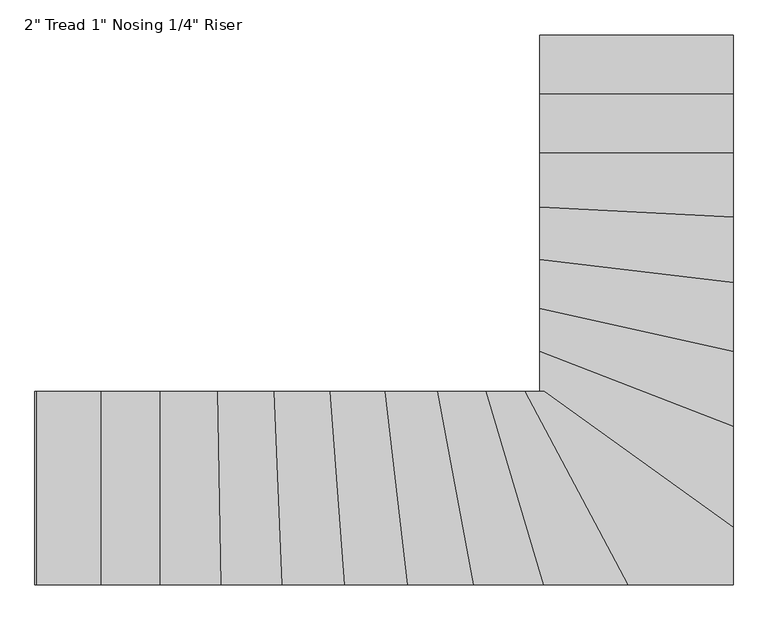
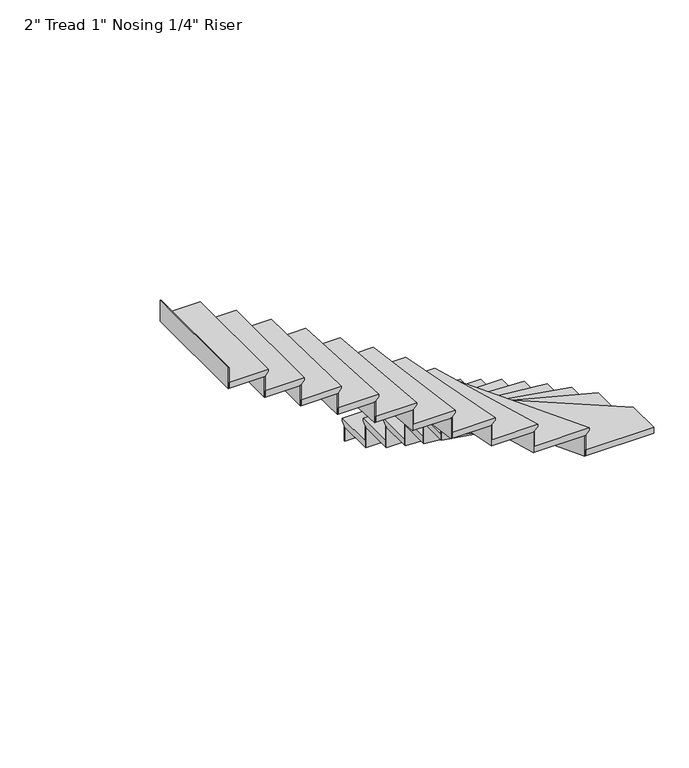
"""IFC4 building model written with IfcOpenShell, lengths in millimetres: stair flight geometry."""

from ifc_helpers import new_model, si_unit, origin, place, context, project, spatial, faceted_brep, source, transform, mapped, element, save


def stair_flight_07df138c(model_context):
    return source(origin(), model_context, "Body", "Brep", [
        faceted_brep([(541.8084916, 3870.4222402, 150.2833333), (541.8084916, 3870.4222402, 169.3333333), (1456.2084916, 3870.4222402, 169.3333333), (1456.2084916, 3870.4222402, 150.2833333), (541.8084916, 3845.0222402, 124.8833333), (1456.2084916, 3845.0222402, 124.8833333), (541.8084916, 3565.6222402, 169.3333333), (1456.2084916, 3565.6222402, 169.3333333), (1456.2084916, 3845.0222402, 118.5333333), (1456.2084916, 3565.6222402, 118.5333333), (541.8084916, 3565.6222402, 118.5333333), (541.8084916, 3845.0222402, 118.5333333)], [[[0, 1, 2, 3]], [[4, 0, 3, 5]], [[2, 1, 6, 7]], [[8, 9, 10, 11]], [[2, 7, 9, 8, 5, 3]], [[8, 11, 4, 5]], [[6, 1, 0, 4, 11, 10]], [[7, 6, 10, 9]]]),
        faceted_brep([(541.8084916, 3845.0222402, 118.5333333), (541.8084916, 3845.0222402, 0.0), (541.8084916, 3838.6722402, 0.0), (541.8084916, 3838.6722402, 118.5333333), (1456.2084916, 3845.0222402, 118.5333333), (1456.2084916, 3838.6722402, 118.5333333), (1456.2084916, 3838.6722402, 0.0), (1456.2084916, 3845.0222402, 0.0)], [[[0, 1, 2, 3]], [[4, 5, 6, 7]], [[1, 0, 4, 7]], [[2, 1, 7, 6]], [[3, 2, 6, 5]], [[0, 3, 5, 4]]]),
        faceted_brep([(541.8084916, 3565.6222402, 287.8666667), (541.8084916, 3565.6222402, 118.5333333), (541.8084916, 3559.2722402, 118.5333333), (541.8084916, 3559.2722402, 287.8666667), (1456.2084916, 3565.6222402, 287.8666667), (1456.2084916, 3559.2722402, 287.8666667), (1456.2084916, 3559.2722402, 118.5333333), (1456.2084916, 3565.6222402, 118.5333333)], [[[0, 1, 2, 3]], [[4, 5, 6, 7]], [[1, 0, 4, 7]], [[2, 1, 7, 6]], [[3, 2, 6, 5]], [[0, 3, 5, 4]]]),
        faceted_brep([(1456.2084916, 3591.0222402, 338.6666667), (541.8084916, 3591.0222402, 338.6666667), (541.8084916, 3286.2222402, 338.6666667), (1456.2084916, 3286.2222402, 338.6666667), (1456.2084916, 3565.6222402, 287.8666667), (1456.2084916, 3286.2222402, 287.8666667), (541.8084916, 3286.2222402, 287.8666667), (541.8084916, 3565.6222402, 287.8666667), (1456.2084916, 3565.6222402, 294.2166667), (1456.2084916, 3591.0222402, 319.6166667), (541.8084916, 3565.6222402, 294.2166667), (541.8084916, 3591.0222402, 319.6166667)], [[[0, 1, 2, 3]], [[4, 5, 6, 7]], [[0, 3, 5, 4, 8, 9]], [[4, 7, 10, 8]], [[2, 1, 11, 10, 7, 6]], [[3, 2, 6, 5]], [[11, 1, 0, 9]], [[10, 11, 9, 8]]]),
        faceted_brep([(541.8084916, 3286.2222402, 457.2), (541.8084916, 3286.2222402, 287.8666667), (541.8084916, 3279.8722402, 287.8666667), (541.8084916, 3279.8722402, 457.2), (1456.2084916, 3286.2222402, 457.2), (1456.2084916, 3279.8722402, 457.2), (1456.2084916, 3279.8722402, 287.8666667), (1456.2084916, 3286.2222402, 287.8666667)], [[[0, 1, 2, 3]], [[4, 5, 6, 7]], [[1, 0, 4, 7]], [[2, 1, 7, 6]], [[3, 2, 6, 5]], [[0, 3, 5, 4]]]),
        faceted_brep([(1456.2084916, 3311.6222402, 508.0), (541.8084916, 3311.6222402, 508.0), (541.8084916, 3029.9557204, 508.0), (1456.2084916, 2983.6235901, 508.0), (1456.2084916, 3286.2222402, 457.2), (1456.2084916, 2983.6235901, 457.2), (541.8084916, 3029.9557204, 457.2), (541.8084916, 3286.2222402, 457.2), (1456.2084916, 3286.2222402, 463.55), (1456.2084916, 3311.6222402, 488.95), (541.8084916, 3286.2222402, 463.55), (541.8084916, 3311.6222402, 488.95)], [[[0, 1, 2, 3]], [[4, 5, 6, 7]], [[0, 3, 5, 4, 8, 9]], [[4, 7, 10, 8]], [[2, 1, 11, 10, 7, 6]], [[3, 2, 6, 5]], [[11, 1, 0, 9]], [[10, 11, 9, 8]]]),
        faceted_brep([(541.8084916, 3029.9557204, 626.5333333), (541.8084916, 3029.9557204, 457.2), (541.8084916, 3023.5975741, 457.2), (541.8084916, 3023.5975741, 626.5333333), (1456.2084916, 2983.6235901, 626.5333333), (1456.2084916, 2977.2654439, 626.5333333), (1456.2084916, 2977.2654439, 457.2), (1456.2084916, 2983.6235901, 457.2)], [[[0, 1, 2, 3]], [[4, 5, 6, 7]], [[1, 0, 4, 7]], [[2, 1, 7, 6]], [[3, 2, 6, 5]], [[0, 3, 5, 4]]]),
        faceted_brep([(1456.2084916, 3009.0561751, 677.3333333), (541.8084916, 3055.3883053, 677.3333333), (541.8084916, 2782.3369776, 677.3333333), (1456.2084916, 2672.1399389, 677.3333333), (1456.2084916, 2983.6235901, 626.5333333), (1456.2084916, 2672.1399389, 626.5333333), (541.8084916, 2782.3369776, 626.5333333), (541.8084916, 3029.9557204, 626.5333333), (1456.2084916, 2983.6235901, 632.8833333), (1456.2084916, 3009.0561751, 658.2833333), (541.8084916, 3029.9557204, 632.8833333), (541.8084916, 3055.3883053, 658.2833333)], [[[0, 1, 2, 3]], [[4, 5, 6, 7]], [[0, 3, 5, 4, 8, 9]], [[4, 7, 10, 8]], [[2, 1, 11, 10, 7, 6]], [[3, 2, 6, 5]], [[11, 1, 0, 9]], [[10, 11, 9, 8]]]),
        faceted_brep([(541.8084916, 2782.3369776, 795.8666667), (541.8084916, 2782.3369776, 626.5333333), (541.8084916, 2775.9410322, 626.5333333), (541.8084916, 2775.9410322, 795.8666667), (1456.2084916, 2672.1399389, 795.8666667), (1456.2084916, 2665.7439934, 795.8666667), (1456.2084916, 2665.7439934, 626.5333333), (1456.2084916, 2672.1399389, 626.5333333)], [[[0, 1, 2, 3]], [[4, 5, 6, 7]], [[1, 0, 4, 7]], [[2, 1, 7, 6]], [[3, 2, 6, 5]], [[0, 3, 5, 4]]]),
        faceted_brep([(1456.2084916, 2697.7237208, 846.6666667), (541.8084916, 2807.9207596, 846.6666667), (541.8084916, 2549.3331683, 846.6666667), (1456.2084916, 2345.4640286, 846.6666667), (1456.2084916, 2672.1399389, 795.8666667), (1456.2084916, 2345.4640286, 795.8666667), (541.8084916, 2549.3331683, 795.8666667), (541.8084916, 2782.3369776, 795.8666667), (1456.2084916, 2672.1399389, 802.2166667), (1456.2084916, 2697.7237208, 827.6166667), (541.8084916, 2782.3369776, 802.2166667), (541.8084916, 2807.9207596, 827.6166667)], [[[0, 1, 2, 3]], [[4, 5, 6, 7]], [[0, 3, 5, 4, 8, 9]], [[4, 7, 10, 8]], [[2, 1, 11, 10, 7, 6]], [[3, 2, 6, 5]], [[11, 1, 0, 9]], [[10, 11, 9, 8]]]),
        faceted_brep([(541.8084916, 2549.3331683, 965.2), (541.8084916, 2549.3331683, 795.8666667), (541.8084916, 2542.8272579, 795.8666667), (541.8084916, 2542.8272579, 965.2), (1456.2084916, 2345.4640286, 965.2), (1456.2084916, 2338.9581182, 965.2), (1456.2084916, 2338.9581182, 795.8666667), (1456.2084916, 2345.4640286, 795.8666667)], [[[0, 1, 2, 3]], [[4, 5, 6, 7]], [[1, 0, 4, 7]], [[2, 1, 7, 6]], [[3, 2, 6, 5]], [[0, 3, 5, 4]]]),
        faceted_brep([(1456.2084916, 2371.4876703, 1016.0), (541.8084916, 2575.3568101, 1016.0), (541.8084916, 2344.0635087, 1016.0), (1456.2084916, 1989.4955623, 1016.0), (1456.2084916, 2345.4640286, 965.2), (1456.2084916, 1989.4955623, 965.2), (541.8084916, 2344.0635087, 965.2), (541.8084916, 2549.3331683, 965.2), (1456.2084916, 2345.4640286, 971.55), (1456.2084916, 2371.4876703, 996.95), (541.8084916, 2549.3331683, 971.55), (541.8084916, 2575.3568101, 996.95)], [[[0, 1, 2, 3]], [[4, 5, 6, 7]], [[0, 3, 5, 4, 8, 9]], [[4, 7, 10, 8]], [[2, 1, 11, 10, 7, 6]], [[3, 2, 6, 5]], [[11, 1, 0, 9]], [[10, 11, 9, 8]]]),
        faceted_brep([(541.8084916, 2344.0635087, 1134.5333333), (541.8084916, 2344.0635087, 965.2), (541.8084916, 2337.2528325, 965.2), (541.8084916, 2337.2528325, 1134.5333333), (1456.2084916, 1989.4955623, 1134.5333333), (1456.2084916, 1982.6848861, 1134.5333333), (1456.2084916, 1982.6848861, 965.2), (1456.2084916, 1989.4955623, 965.2)], [[[0, 1, 2, 3]], [[4, 5, 6, 7]], [[1, 0, 4, 7]], [[2, 1, 7, 6]], [[3, 2, 6, 5]], [[0, 3, 5, 4]]]),
        faceted_brep([(1456.2084916, 2016.738267, 1185.3333333), (541.8084916, 2371.3062134, 1185.3333333), (541.8084916, 2183.3652728, 1185.3333333), (518.7146085, 2183.3652728, 1185.3333333), (1456.2084916, 1508.8170155, 1185.3333333), (1456.2084916, 1989.4955623, 1134.5333333), (1456.2084916, 1508.8170155, 1134.5333333), (518.7146085, 2183.3652728, 1134.5333333), (541.8084916, 2183.3652728, 1134.5333333), (541.8084916, 2344.0635087, 1134.5333333), (1456.2084916, 1989.4955623, 1140.8833333), (1456.2084916, 2016.738267, 1166.2833333), (541.8084916, 2344.0635087, 1140.8833333), (541.8084916, 2371.3062134, 1166.2833333)], [[[0, 1, 2, 3, 4]], [[5, 6, 7, 8, 9]], [[0, 4, 6, 5, 10, 11]], [[5, 9, 12, 10]], [[2, 1, 13, 12, 9, 8]], [[4, 3, 7, 6]], [[13, 1, 0, 11]], [[12, 13, 11, 10]], [[3, 2, 8, 7]]]),
        faceted_brep([(518.7146085, 2183.3652728, 1303.8666667), (518.7146085, 2183.3652728, 1134.5333333), (507.8422444, 2183.3652728, 1134.5333333), (507.8422444, 2183.3652728, 1303.8666667), (1456.2084916, 1508.8170155, 1303.8666667), (1456.2084916, 1500.9941013, 1303.8666667), (1456.2084916, 1500.9941013, 1134.5333333), (1456.2084916, 1508.8170155, 1134.5333333)], [[[0, 1, 2, 3]], [[4, 5, 6, 7]], [[1, 0, 4, 7]], [[2, 1, 7, 6]], [[3, 2, 6, 5]], [[0, 3, 5, 4]]]),
        faceted_brep([(928.7056408, 1268.9652728, 1354.6666667), (1456.2084916, 1268.9652728, 1354.6666667), (1456.2084916, 1540.1086724, 1354.6666667), (562.2040648, 2183.3652728, 1354.6666667), (442.5531734, 2183.3652728, 1354.6666667), (1456.2084916, 1268.9652728, 1303.8666667), (928.7056408, 1268.9652728, 1303.8666667), (442.5531734, 2183.3652728, 1303.8666667), (518.7146085, 2183.3652728, 1303.8666667), (1456.2084916, 1508.8170155, 1303.8666667), (518.7146085, 2183.3652728, 1310.2166667), (1456.2084916, 1508.8170155, 1310.2166667), (562.2040648, 2183.3652728, 1335.6166667), (1456.2084916, 1540.1086724, 1335.6166667)], [[[0, 1, 2, 3, 4]], [[5, 6, 7, 8, 9]], [[1, 0, 6, 5]], [[9, 8, 10, 11]], [[0, 4, 7, 6]], [[12, 3, 2, 13]], [[10, 12, 13, 11]], [[2, 1, 5, 9, 11, 13]], [[4, 3, 12, 10, 8, 7]]]),
        faceted_brep([(442.5531734, 2183.3652728, 1473.2), (442.5531734, 2183.3652728, 1303.8666667), (435.3614926, 2183.3652728, 1303.8666667), (435.3614926, 2183.3652728, 1473.2), (928.7056408, 1268.9652728, 1473.2), (921.51396, 1268.9652728, 1473.2), (921.51396, 1268.9652728, 1303.8666667), (928.7056408, 1268.9652728, 1303.8666667)], [[[0, 1, 2, 3]], [[4, 5, 6, 7]], [[1, 0, 4, 7]], [[2, 1, 7, 6]], [[3, 2, 6, 5]], [[0, 3, 5, 4]]]),
        faceted_brep([(957.4723641, 1268.9652728, 1524.0), (471.3198967, 2183.3652728, 1524.0), (259.1852093, 2183.3652728, 1524.0), (530.810737, 1268.9652728, 1524.0), (928.7056408, 1268.9652728, 1473.2), (530.810737, 1268.9652728, 1473.2), (259.1852093, 2183.3652728, 1473.2), (442.5531734, 2183.3652728, 1473.2), (928.7056408, 1268.9652728, 1479.55), (957.4723641, 1268.9652728, 1504.95), (442.5531734, 2183.3652728, 1479.55), (471.3198967, 2183.3652728, 1504.95)], [[[0, 1, 2, 3]], [[4, 5, 6, 7]], [[0, 3, 5, 4, 8, 9]], [[4, 7, 10, 8]], [[2, 1, 11, 10, 7, 6]], [[3, 2, 6, 5]], [[11, 1, 0, 9]], [[10, 11, 9, 8]]]),
        faceted_brep([(259.1852093, 2183.3652728, 1642.5333333), (259.1852093, 2183.3652728, 1473.2), (252.5609672, 2183.3652728, 1473.2), (252.5609672, 2183.3652728, 1642.5333333), (530.810737, 1268.9652728, 1642.5333333), (524.1864949, 1268.9652728, 1642.5333333), (524.1864949, 1268.9652728, 1473.2), (530.810737, 1268.9652728, 1473.2)], [[[0, 1, 2, 3]], [[4, 5, 6, 7]], [[1, 0, 4, 7]], [[2, 1, 7, 6]], [[3, 2, 6, 5]], [[0, 3, 5, 4]]]),
        faceted_brep([(557.3077055, 1268.9652728, 1693.3333333), (285.6821779, 2183.3652728, 1693.3333333), (32.036519, 2183.3652728, 1693.3333333), (200.498444, 1268.9652728, 1693.3333333), (530.810737, 1268.9652728, 1642.5333333), (200.498444, 1268.9652728, 1642.5333333), (32.036519, 2183.3652728, 1642.5333333), (259.1852093, 2183.3652728, 1642.5333333), (530.810737, 1268.9652728, 1648.8833333), (557.3077055, 1268.9652728, 1674.2833333), (259.1852093, 2183.3652728, 1648.8833333), (285.6821779, 2183.3652728, 1674.2833333)], [[[0, 1, 2, 3]], [[4, 5, 6, 7]], [[0, 3, 5, 4, 8, 9]], [[4, 7, 10, 8]], [[2, 1, 11, 10, 7, 6]], [[3, 2, 6, 5]], [[11, 1, 0, 9]], [[10, 11, 9, 8]]]),
        faceted_brep([(32.036519, 2183.3652728, 1811.8666667), (32.036519, 2183.3652728, 1642.5333333), (25.579654, 2183.3652728, 1642.5333333), (25.579654, 2183.3652728, 1811.8666667), (200.498444, 1268.9652728, 1811.8666667), (194.0415789, 1268.9652728, 1811.8666667), (194.0415789, 1268.9652728, 1642.5333333), (200.498444, 1268.9652728, 1642.5333333)], [[[0, 1, 2, 3]], [[4, 5, 6, 7]], [[1, 0, 4, 7]], [[2, 1, 7, 6]], [[3, 2, 6, 5]], [[0, 3, 5, 4]]]),
        faceted_brep([(226.3259042, 1268.9652728, 1862.6666667), (57.8639792, 2183.3652728, 1862.6666667), (-216.5399099, 2183.3652728, 1862.6666667), (-109.2188993, 1268.9652728, 1862.6666667), (200.498444, 1268.9652728, 1811.8666667), (-109.2188993, 1268.9652728, 1811.8666667), (-216.5399099, 2183.3652728, 1811.8666667), (32.036519, 2183.3652728, 1811.8666667), (200.498444, 1268.9652728, 1818.2166667), (226.3259042, 1268.9652728, 1843.6166667), (32.036519, 2183.3652728, 1818.2166667), (57.8639792, 2183.3652728, 1843.6166667)], [[[0, 1, 2, 3]], [[4, 5, 6, 7]], [[0, 3, 5, 4, 8, 9]], [[4, 7, 10, 8]], [[2, 1, 11, 10, 7, 6]], [[3, 2, 6, 5]], [[11, 1, 0, 9]], [[10, 11, 9, 8]]]),
        faceted_brep([(-216.5399099, 2183.3652728, 1981.2), (-216.5399099, 2183.3652728, 1811.8666667), (-222.9334965, 2183.3652728, 1811.8666667), (-222.9334965, 2183.3652728, 1981.2), (-109.2188993, 1268.9652728, 1981.2), (-115.6124859, 1268.9652728, 1981.2), (-115.6124859, 1268.9652728, 1811.8666667), (-109.2188993, 1268.9652728, 1811.8666667)], [[[0, 1, 2, 3]], [[4, 5, 6, 7]], [[1, 0, 4, 7]], [[2, 1, 7, 6]], [[3, 2, 6, 5]], [[0, 3, 5, 4]]]),
        faceted_brep([(-83.644553, 1268.9652728, 2032.0), (-190.9655636, 2183.3652728, 2032.0), (-475.6084446, 2183.3652728, 2032.0), (-408.7373342, 1268.9652728, 2032.0), (-109.2188993, 1268.9652728, 1981.2), (-408.7373342, 1268.9652728, 1981.2), (-475.6084446, 2183.3652728, 1981.2), (-216.5399099, 2183.3652728, 1981.2), (-109.2188993, 1268.9652728, 1987.55), (-83.644553, 1268.9652728, 2012.95), (-216.5399099, 2183.3652728, 1987.55), (-190.9655636, 2183.3652728, 2012.95)], [[[0, 1, 2, 3]], [[4, 5, 6, 7]], [[0, 3, 5, 4, 8, 9]], [[4, 7, 10, 8]], [[2, 1, 11, 10, 7, 6]], [[3, 2, 6, 5]], [[11, 1, 0, 9]], [[10, 11, 9, 8]]]),
        faceted_brep([(-475.6084446, 2183.3652728, 2150.5333333), (-475.6084446, 2183.3652728, 1981.2), (-481.9754023, 2183.3652728, 1981.2), (-481.9754023, 2183.3652728, 2150.5333333), (-408.7373342, 1268.9652728, 2150.5333333), (-415.104292, 1268.9652728, 2150.5333333), (-415.104292, 1268.9652728, 1981.2), (-408.7373342, 1268.9652728, 1981.2)], [[[0, 1, 2, 3]], [[4, 5, 6, 7]], [[1, 0, 4, 7]], [[2, 1, 7, 6]], [[3, 2, 6, 5]], [[0, 3, 5, 4]]]),
        faceted_brep([(-383.2695031, 1268.9652728, 2201.3333333), (-450.1406135, 2183.3652728, 2201.3333333), (-740.5916411, 2183.3652728, 2201.3333333), (-702.4626207, 1268.9652728, 2201.3333333), (-408.7373342, 1268.9652728, 2150.5333333), (-702.4626207, 1268.9652728, 2150.5333333), (-740.5916411, 2183.3652728, 2150.5333333), (-475.6084446, 2183.3652728, 2150.5333333), (-408.7373342, 1268.9652728, 2156.8833333), (-383.2695031, 1268.9652728, 2182.2833333), (-475.6084446, 2183.3652728, 2156.8833333), (-450.1406135, 2183.3652728, 2182.2833333)], [[[0, 1, 2, 3]], [[4, 5, 6, 7]], [[0, 3, 5, 4, 8, 9]], [[4, 7, 10, 8]], [[2, 1, 11, 10, 7, 6]], [[3, 2, 6, 5]], [[11, 1, 0, 9]], [[10, 11, 9, 8]]]),
        faceted_brep([(-740.5916411, 2183.3652728, 2319.8666667), (-740.5916411, 2183.3652728, 2150.5333333), (-746.9471593, 2183.3652728, 2150.5333333), (-746.9471593, 2183.3652728, 2319.8666667), (-702.4626207, 1268.9652728, 2319.8666667), (-708.8181389, 1268.9652728, 2319.8666667), (-708.8181389, 1268.9652728, 2150.5333333), (-702.4626207, 1268.9652728, 2150.5333333)], [[[0, 1, 2, 3]], [[4, 5, 6, 7]], [[1, 0, 4, 7]], [[2, 1, 7, 6]], [[3, 2, 6, 5]], [[0, 3, 5, 4]]]),
        faceted_brep([(-677.0405481, 1268.9652728, 2370.6666667), (-715.1695685, 2183.3652728, 2370.6666667), (-1009.2364216, 2183.3652728, 2370.6666667), (-992.5821201, 1268.9652728, 2370.6666667), (-702.4626207, 1268.9652728, 2319.8666667), (-992.5821201, 1268.9652728, 2319.8666667), (-1009.2364216, 2183.3652728, 2319.8666667), (-740.5916411, 2183.3652728, 2319.8666667), (-702.4626207, 1268.9652728, 2326.2166667), (-677.0405481, 1268.9652728, 2351.6166667), (-740.5916411, 2183.3652728, 2326.2166667), (-715.1695685, 2183.3652728, 2351.6166667)], [[[0, 1, 2, 3]], [[4, 5, 6, 7]], [[0, 3, 5, 4, 8, 9]], [[4, 7, 10, 8]], [[2, 1, 11, 10, 7, 6]], [[3, 2, 6, 5]], [[11, 1, 0, 9]], [[10, 11, 9, 8]]]),
        faceted_brep([(-1009.2364216, 2183.3652728, 2489.2), (-1009.2364216, 2183.3652728, 2319.8666667), (-1015.5874748, 2183.3652728, 2319.8666667), (-1015.5874748, 2183.3652728, 2489.2), (-992.5821201, 1268.9652728, 2489.2), (-998.9331733, 1268.9652728, 2489.2), (-998.9331733, 1268.9652728, 2319.8666667), (-992.5821201, 1268.9652728, 2319.8666667)], [[[0, 1, 2, 3]], [[4, 5, 6, 7]], [[1, 0, 4, 7]], [[2, 1, 7, 6]], [[3, 2, 6, 5]], [[0, 3, 5, 4]]]),
        faceted_brep([(-967.1779075, 1268.9652728, 2540.0), (-983.832209, 2183.3652728, 2540.0), (-1280.3050583, 2183.3652728, 2540.0), (-1280.3050583, 1268.9652728, 2540.0), (-992.5821201, 1268.9652728, 2489.2), (-1280.3050583, 1268.9652728, 2489.2), (-1280.3050583, 2183.3652728, 2489.2), (-1009.2364216, 2183.3652728, 2489.2), (-992.5821201, 1268.9652728, 2495.55), (-967.1779075, 1268.9652728, 2520.95), (-1009.2364216, 2183.3652728, 2495.55), (-983.832209, 2183.3652728, 2520.95)], [[[0, 1, 2, 3]], [[4, 5, 6, 7]], [[0, 3, 5, 4, 8, 9]], [[4, 7, 10, 8]], [[2, 1, 11, 10, 7, 6]], [[3, 2, 6, 5]], [[11, 1, 0, 9]], [[10, 11, 9, 8]]]),
        faceted_brep([(-1280.3050583, 2183.3652728, 2658.5333333), (-1280.3050583, 2183.3652728, 2489.2), (-1286.6550583, 2183.3652728, 2489.2), (-1286.6550583, 2183.3652728, 2658.5333333), (-1280.3050583, 1268.9652728, 2658.5333333), (-1286.6550583, 1268.9652728, 2658.5333333), (-1286.6550583, 1268.9652728, 2489.2), (-1280.3050583, 1268.9652728, 2489.2)], [[[0, 1, 2, 3]], [[4, 5, 6, 7]], [[1, 0, 4, 7]], [[2, 1, 7, 6]], [[3, 2, 6, 5]], [[0, 3, 5, 4]]]),
        faceted_brep([(-1254.9050583, 1268.9652728, 2709.3333333), (-1254.9050583, 2183.3652728, 2709.3333333), (-1559.7050583, 2183.3652728, 2709.3333333), (-1559.7050583, 1268.9652728, 2709.3333333), (-1280.3050583, 1268.9652728, 2658.5333333), (-1559.7050583, 1268.9652728, 2658.5333333), (-1559.7050583, 2183.3652728, 2658.5333333), (-1280.3050583, 2183.3652728, 2658.5333333), (-1280.3050583, 1268.9652728, 2664.8833333), (-1254.9050583, 1268.9652728, 2690.2833333), (-1280.3050583, 2183.3652728, 2664.8833333), (-1254.9050583, 2183.3652728, 2690.2833333)], [[[0, 1, 2, 3]], [[4, 5, 6, 7]], [[0, 3, 5, 4, 8, 9]], [[4, 7, 10, 8]], [[2, 1, 11, 10, 7, 6]], [[3, 2, 6, 5]], [[11, 1, 0, 9]], [[10, 11, 9, 8]]]),
        faceted_brep([(-1559.7050583, 2183.3652728, 2827.8666667), (-1559.7050583, 2183.3652728, 2658.5333333), (-1566.0550583, 2183.3652728, 2658.5333333), (-1566.0550583, 2183.3652728, 2827.8666667), (-1559.7050583, 1268.9652728, 2827.8666667), (-1566.0550583, 1268.9652728, 2827.8666667), (-1566.0550583, 1268.9652728, 2658.5333333), (-1559.7050583, 1268.9652728, 2658.5333333)], [[[0, 1, 2, 3]], [[4, 5, 6, 7]], [[1, 0, 4, 7]], [[2, 1, 7, 6]], [[3, 2, 6, 5]], [[0, 3, 5, 4]]]),
        faceted_brep([(-1839.1050583, 2183.3652728, 2997.2), (-1839.1050583, 2183.3652728, 2827.8666667), (-1845.4550583, 2183.3652728, 2827.8666667), (-1845.4550583, 2183.3652728, 2997.2), (-1839.1050583, 1268.9652728, 2997.2), (-1845.4550583, 1268.9652728, 2997.2), (-1845.4550583, 1268.9652728, 2827.8666667), (-1839.1050583, 1268.9652728, 2827.8666667)], [[[0, 1, 2, 3]], [[4, 5, 6, 7]], [[1, 0, 4, 7]], [[2, 1, 7, 6]], [[3, 2, 6, 5]], [[0, 3, 5, 4]]]),
        faceted_brep([(-1534.3050583, 1268.9652728, 2878.6666667), (-1534.3050583, 2183.3652728, 2878.6666667), (-1839.1050583, 2183.3652728, 2878.6666667), (-1839.1050583, 1268.9652728, 2878.6666667), (-1559.7050583, 1268.9652728, 2827.8666667), (-1839.1050583, 1268.9652728, 2827.8666667), (-1839.1050583, 2183.3652728, 2827.8666667), (-1559.7050583, 2183.3652728, 2827.8666667), (-1559.7050583, 1268.9652728, 2834.2166667), (-1534.3050583, 1268.9652728, 2859.6166667), (-1559.7050583, 2183.3652728, 2834.2166667), (-1534.3050583, 2183.3652728, 2859.6166667)], [[[0, 1, 2, 3]], [[4, 5, 6, 7]], [[0, 3, 5, 4, 8, 9]], [[4, 7, 10, 8]], [[2, 1, 11, 10, 7, 6]], [[3, 2, 6, 5]], [[11, 1, 0, 9]], [[10, 11, 9, 8]]]),
    ])


if __name__ == "__main__":
    model = new_model("IFC4")
    model_context = context("Model", 3, world=origin())
    ifc_project = project(units=[si_unit("LENGTHUNIT", "METRE", prefix="MILLI")], contexts=[model_context])
    site = spatial("IfcSite", under=ifc_project)
    building = spatial("IfcBuilding", under=site)
    placement = place(None, origin())
    stair_flight_shape = stair_flight_07df138c(model_context)
    element("IfcStairFlight", 1, ObjectType="2\" Tread 1\" Nosing 1/4\" Riser", at=placement, inside=building, context=model_context, shape_type="MappedRepresentation", body=[
        mapped(stair_flight_shape, transform((0.0, 0.0, 0.0), x_axis=(1.0, 0.0, 0.0), y_axis=(0.0, 1.0, 0.0), z_axis=(0.0, 0.0, 1.0))),
    ])
    save(model, "model.ifc")
